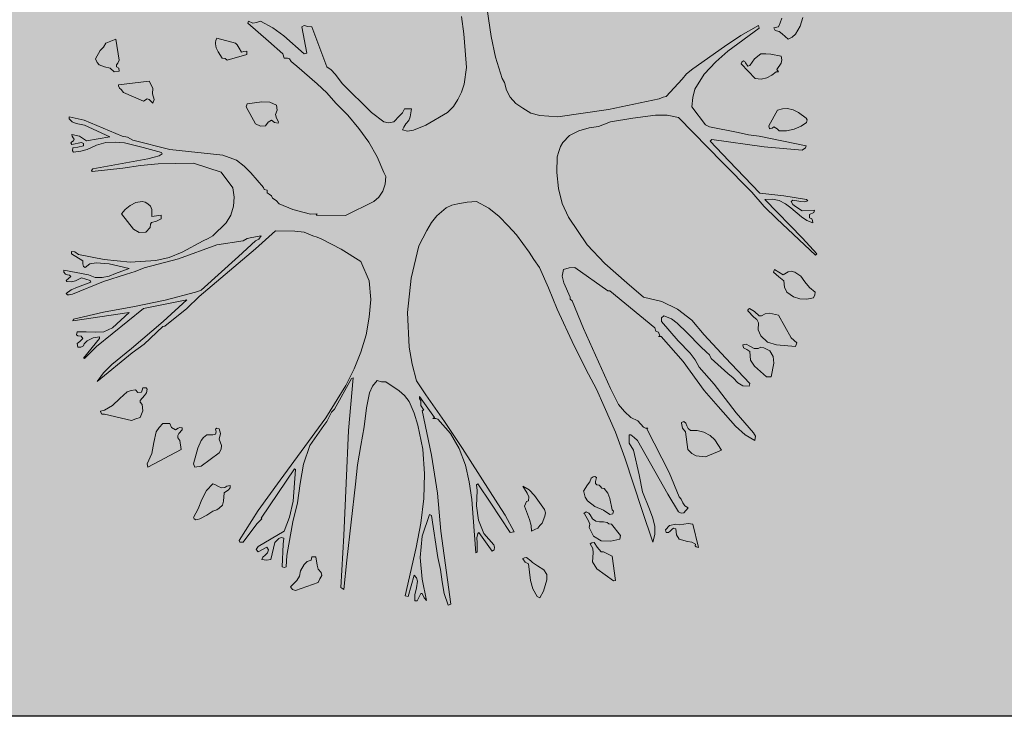
# Model space of a CAD drawing. Units: inches. Extents: x 84 to 1044, y -280 to 906.
# Tile 35 of 105: x 848 to 876, y -113 to -93. Entities that reach past the tile are written whole.
import ezdxf

# ---------------------------------------------------------------- set-up
doc = ezdxf.new("R2010")
doc.units = ezdxf.units.IN
doc.layers.add('C-PROP', color=7, linetype='Continuous', lineweight=25)
doc.layers.add('L-PLNT', color=114, linetype='Continuous', lineweight=15)
doc.layers.add('L-PLNT-PATT', color=9, linetype='Continuous', lineweight=9, true_color=0xafd9aa)

# ---------------------------------------------------------------- blocks, each defined once
blk = doc.blocks.new('A$C37E508DF')
for p, q in [((0.7911, 1.1436), (0.8027, 1.0677)), ((0.3456, 1.093), (0.3469, 1.0964)), ((0.3842, 1.0591), (0.3456, 1.093)), ((0.3469, 1.0964), (0.355, 1.093)), ((0.355, 1.093), (0.3619, 1.0943)), ((0.3619, 1.0943), (0.3692, 1.0968)), ((0.3692, 1.0968), (0.3923, 1.0844)), ((0.7512, 1.0728), (0.7469, 1.1054)), ((1.3421, 1.0861), (1.3455, 1.0934)), ((1.3455, 1.0934), (1.3485, 1.102)), ((1.3875, 1.1037), (1.3828, 1.087)), ((0.3923, 1.0844), (0.4129, 1.069)), ((0.4472, 1.0857), (0.4515, 1.0887)), ((0.4562, 1.0364), (0.4472, 1.0857)), ((0.4515, 1.0887), (0.4584, 1.0865)), ((0.4584, 1.0865), (0.4657, 1.0861)), ((0.4657, 1.0861), (0.4939, 1.0107)), ((0.7538, 1.0415), (0.7512, 1.0728)), ((1.3057, 1.0835), (1.2469, 1.0402)), ((1.2713, 1.0694), (1.3044, 1.0887)), ((1.3044, 1.0887), (1.3057, 1.0835)), ((1.3335, 1.0844), (1.3421, 1.0861)), ((1.3361, 1.0793), (1.3335, 1.0844)), ((1.3434, 1.0771), (1.3361, 1.0793)), ((1.349, 1.0728), (1.3434, 1.0771)), ((1.3605, 1.063), (1.349, 1.0728)), ((1.3828, 1.087), (1.3738, 1.072)), ((0.0746, 1.0475), (0.0789, 1.0552)), ((0.0789, 1.0552), (0.0978, 1.063)), ((0.0978, 1.063), (0.1042, 1.0231)), ((0.2847, 1.0565), (0.2856, 1.0604)), ((0.2851, 1.054), (0.2847, 1.0565)), ((0.2864, 1.0463), (0.2851, 1.054)), ((0.2856, 1.0604), (0.2877, 1.0647)), ((0.2877, 1.0647), (0.3224, 1.0552)), ((0.3224, 1.0552), (0.3255, 1.0522)), ((0.4112, 1.0351), (0.3842, 1.0591)), ((0.4129, 1.069), (0.4515, 1.0351)), ((0.8027, 1.0677), (0.8108, 1.0287)), ((1.2409, 1.0488), (1.2713, 1.0694)), ((1.3678, 1.0664), (1.3605, 1.063)), ((1.3738, 1.072), (1.3678, 1.0664)), ((0.0596, 1.0257), (0.0682, 1.0415)), ((0.0682, 1.0415), (0.0746, 1.0475)), ((0.2899, 1.039), (0.2864, 1.0463)), ((0.2972, 1.0274), (0.2899, 1.039)), ((0.3255, 1.0522), (0.3293, 1.0458)), ((0.3293, 1.0458), (0.3336, 1.0381)), ((0.3336, 1.0381), (0.3383, 1.0398)), ((0.3383, 1.0398), (0.3439, 1.0402)), ((0.3439, 1.0402), (0.3439, 1.0338)), ((0.4515, 1.0351), (0.4562, 1.0364)), ((0.7559, 1.0098), (0.7538, 1.0415)), ((1.1813, 1.0072), (1.2409, 1.0488)), ((1.2469, 1.0402), (1.2246, 1.0201)), ((1.3091, 1.0351), (1.3185, 1.0355)), ((1.3185, 1.0355), (1.3275, 1.0347)), ((0.0626, 1.0188), (0.0596, 1.0257)), ((0.0665, 1.0149), (0.0626, 1.0188)), ((0.1012, 1.018), (0.099, 1.0149)), ((0.1042, 1.0231), (0.1012, 1.018)), ((0.3032, 1.0265), (0.2972, 1.0274)), ((0.3066, 1.0231), (0.3032, 1.0265)), ((0.3439, 1.0338), (0.3066, 1.0231)), ((0.4138, 1.0274), (0.4112, 1.0351)), ((0.4202, 1.0274), (0.4138, 1.0274)), ((0.4241, 1.0257), (0.4202, 1.0274)), ((0.4267, 1.0209), (0.4241, 1.0257)), ((0.4305, 1.0175), (0.4267, 1.0209)), ((0.4378, 1.0124), (0.4305, 1.0175)), ((0.8108, 1.0287), (0.8233, 0.9892)), ((1.2246, 1.0201), (1.2023, 0.9969)), ((1.2718, 1.0162), (1.2731, 1.0197)), ((1.2731, 1.0197), (1.2761, 1.0218)), ((1.2761, 1.0218), (1.2786, 1.0209)), ((1.2786, 1.0209), (1.2799, 1.0184)), ((1.2799, 1.0184), (1.2842, 1.0124)), ((1.2885, 1.0136), (1.2971, 1.0257)), ((1.2971, 1.0257), (1.3091, 1.0351)), ((1.3275, 1.0347), (1.3468, 1.0308)), ((1.3468, 1.018), (1.3391, 1.0059)), ((1.3468, 1.0308), (1.3481, 1.0239)), ((1.3481, 1.0239), (1.3468, 1.018)), ((0.0763, 1.0111), (0.0665, 1.0149)), ((0.087, 1.0085), (0.0763, 1.0111)), ((0.0948, 1.0016), (0.087, 1.0085)), ((0.1042, 1.0029), (0.0948, 1.0016)), ((0.099, 1.0149), (0.099, 1.0111)), ((0.099, 1.0111), (0.1033, 1.0085)), ((0.1033, 1.0085), (0.1042, 1.0029)), ((0.476, 0.9789), (0.4378, 1.0124)), ((0.4939, 1.0107), (0.5021, 1.0051)), ((0.5021, 1.0051), (0.5094, 0.9969)), ((0.7516, 0.9785), (0.7559, 1.0098)), ((1.1693, 0.9974), (1.1813, 1.0072)), ((1.2984, 0.9892), (1.2718, 1.0162)), ((1.2842, 1.0124), (1.2885, 1.0136)), ((1.3378, 1.0016), (1.3297, 0.9952)), ((1.3421, 1.0016), (1.3378, 1.0016)), ((1.3391, 1.0059), (1.3421, 1.0016)), ((0.1029, 0.9772), (0.1604, 0.9841)), ((0.1604, 0.9841), (0.1672, 0.9708)), ((0.5094, 0.9969), (0.5231, 0.9789)), ((0.8233, 0.9892), (0.8275, 0.9815)), ((0.8275, 0.9815), (0.8314, 0.9673)), ((1.1311, 0.9549), (1.1612, 0.9879)), ((1.1612, 0.9879), (1.1693, 0.9974)), ((1.2023, 0.9969), (1.1852, 0.9691)), ((1.3095, 0.9875), (1.2984, 0.9892)), ((1.3202, 0.9901), (1.3095, 0.9875)), ((1.3297, 0.9952), (1.3202, 0.9901)), ((0.1025, 0.9751), (0.1029, 0.9772)), ((0.1046, 0.9708), (0.1025, 0.9751)), ((0.1076, 0.9682), (0.1046, 0.9708)), ((0.1119, 0.9626), (0.1076, 0.9682)), ((0.1496, 0.9463), (0.1119, 0.9626)), ((0.1672, 0.9708), (0.1664, 0.9601)), ((0.4939, 0.9618), (0.476, 0.9789)), ((0.5111, 0.9429), (0.4939, 0.9618)), ((0.5231, 0.9789), (0.578, 0.9253)), ((0.7401, 0.9493), (0.7469, 0.9635)), ((0.7469, 0.9635), (0.7516, 0.9785)), ((0.8314, 0.9673), (0.8383, 0.954)), ((1.1852, 0.9691), (1.1809, 0.9532)), ((0.1565, 0.9506), (0.1496, 0.9463)), ((0.1604, 0.9493), (0.1565, 0.9506)), ((0.1629, 0.9468), (0.1604, 0.9493)), ((0.1672, 0.9429), (0.1629, 0.9468)), ((0.1664, 0.9601), (0.1698, 0.9493)), ((0.1698, 0.9493), (0.1672, 0.9429)), ((0.3443, 0.9412), (0.3722, 0.9451)), ((0.3722, 0.9451), (0.3868, 0.9446)), ((0.3868, 0.9446), (0.3992, 0.9386)), ((0.7315, 0.9365), (0.7401, 0.9493)), ((0.8383, 0.954), (0.8486, 0.942)), ((1.0227, 0.9309), (1.1183, 0.9506)), ((1.1183, 0.9506), (1.1256, 0.954)), ((1.1256, 0.954), (1.1311, 0.9549)), ((1.1809, 0.9532), (1.1796, 0.936)), ((0.3426, 0.936), (0.3443, 0.9412)), ((0.3602, 0.9039), (0.3426, 0.936)), ((0.4009, 0.9292), (0.3975, 0.9215)), ((0.3992, 0.9386), (0.4009, 0.9292)), ((0.5334, 0.9202), (0.5111, 0.9429)), ((0.578, 0.9253), (0.6011, 0.9077)), ((0.6303, 0.9189), (0.6359, 0.9245)), ((0.6359, 0.9245), (0.6397, 0.9322)), ((0.6397, 0.9322), (0.653, 0.9322)), ((0.653, 0.9322), (0.6505, 0.9172)), ((0.6796, 0.9013), (0.7203, 0.9253)), ((0.7203, 0.9253), (0.7315, 0.9365)), ((0.8486, 0.942), (0.8619, 0.933)), ((0.8619, 0.933), (0.8769, 0.9236)), ((0.9279, 0.9172), (1.0227, 0.9309)), ((1.1796, 0.936), (1.2049, 0.9022)), ((1.3241, 0.9), (1.3404, 0.9292)), ((1.3404, 0.9292), (1.3494, 0.9322)), ((1.3494, 0.9322), (1.3592, 0.9326)), ((1.3592, 0.9326), (1.3695, 0.93)), ((1.3695, 0.93), (1.3794, 0.9253)), ((1.3794, 0.9253), (1.394, 0.9146)), ((0.0103, 0.9129), (0.0103, 0.9172)), ((0.0103, 0.9172), (0.0382, 0.9107)), ((0.0159, 0.9073), (0.0103, 0.9129)), ((0.0232, 0.9043), (0.0159, 0.9073)), ((0.0382, 0.9107), (0.1098, 0.8807)), ((0.3838, 0.9069), (0.379, 0.9)), ((0.3898, 0.9107), (0.3838, 0.9069)), ((0.3958, 0.906), (0.3898, 0.9107)), ((0.4026, 0.9052), (0.3958, 0.906)), ((0.3975, 0.9215), (0.3996, 0.9142)), ((0.3996, 0.9142), (0.4031, 0.9077)), ((0.4031, 0.9077), (0.4026, 0.9052)), ((0.554, 0.8953), (0.5334, 0.9202)), ((0.6011, 0.9077), (0.6097, 0.9056)), ((0.6097, 0.9056), (0.6196, 0.9077)), ((0.6196, 0.9077), (0.6303, 0.9189)), ((0.6479, 0.9103), (0.6423, 0.9039)), ((0.6505, 0.9172), (0.6479, 0.9103)), ((0.8769, 0.9236), (0.8936, 0.9193)), ((0.8936, 0.9193), (0.9279, 0.9172)), ((1.0269, 0.9077), (1.0042, 0.8987)), ((1.0685, 0.9142), (1.0269, 0.9077)), ((1.1114, 0.9198), (1.0685, 0.9142)), ((1.1333, 0.9202), (1.1114, 0.9198)), ((1.1543, 0.9159), (1.1333, 0.9202)), ((1.2371, 0.8314), (1.1543, 0.9159)), ((1.3948, 0.9065), (1.3846, 0.8992)), ((1.394, 0.9146), (1.3957, 0.9112)), ((1.3957, 0.9112), (1.3948, 0.9065)), ((0.0386, 0.9013), (0.0232, 0.9043)), ((0.0866, 0.8794), (0.0386, 0.9013)), ((0.3692, 0.8992), (0.3602, 0.9039)), ((0.379, 0.9), (0.3692, 0.8992)), ((0.5728, 0.8691), (0.554, 0.8953)), ((0.6384, 0.8974), (0.6359, 0.8927)), ((0.6359, 0.8927), (0.6457, 0.8897)), ((0.6423, 0.9039), (0.6384, 0.8974)), ((0.6457, 0.8897), (0.6569, 0.8919)), ((0.6569, 0.8919), (0.6796, 0.9013)), ((0.9673, 0.8906), (0.9498, 0.8816)), ((0.9866, 0.8962), (0.9673, 0.8906)), ((1.0042, 0.8987), (0.9866, 0.8962)), ((1.2049, 0.9022), (1.2126, 0.8983)), ((1.2126, 0.8983), (1.2662, 0.8876)), ((1.2662, 0.8876), (1.2855, 0.8833)), ((1.3254, 0.8944), (1.3241, 0.9)), ((1.3301, 0.8957), (1.3254, 0.8944)), ((1.3335, 0.8983), (1.3301, 0.8957)), ((1.3395, 0.8944), (1.3335, 0.8983)), ((1.3434, 0.8906), (1.3395, 0.8944)), ((1.3571, 0.8906), (1.3434, 0.8906)), ((1.3713, 0.8936), (1.3571, 0.8906)), ((1.3846, 0.8992), (1.3713, 0.8936)), ((0.0133, 0.8679), (0.015, 0.87)), ((0.015, 0.87), (0.0184, 0.8717)), ((0.0159, 0.8803), (0.0154, 0.8837)), ((0.0154, 0.8837), (0.0292, 0.8803)), ((0.0176, 0.8777), (0.0159, 0.8803)), ((0.0193, 0.8752), (0.0176, 0.8777)), ((0.0184, 0.8717), (0.0193, 0.8752)), ((0.0292, 0.8803), (0.0424, 0.8717)), ((0.0424, 0.8717), (0.0866, 0.8794)), ((0.0965, 0.8696), (0.0789, 0.8687)), ((0.1141, 0.8679), (0.0965, 0.8696)), ((0.1098, 0.8807), (0.1196, 0.8786)), ((0.1196, 0.8786), (0.1295, 0.873)), ((0.1295, 0.873), (0.1994, 0.8554)), ((0.5887, 0.8421), (0.5728, 0.8691)), ((0.9498, 0.8816), (0.9369, 0.8687)), ((1.2169, 0.8743), (1.2135, 0.8713)), ((1.2135, 0.8713), (1.2491, 0.834)), ((1.3151, 0.8606), (1.2169, 0.8743)), ((1.2855, 0.8833), (1.3057, 0.8807)), ((1.3057, 0.8807), (1.394, 0.8623)), ((0.0154, 0.8649), (0.0133, 0.8679)), ((0.0334, 0.8687), (0.0154, 0.8649)), ((0.0163, 0.8529), (0.0171, 0.8584)), ((0.0184, 0.8503), (0.0163, 0.8529)), ((0.0171, 0.8584), (0.0266, 0.8602)), ((0.0317, 0.8524), (0.0184, 0.8503)), ((0.0266, 0.8602), (0.0369, 0.8623)), ((0.0442, 0.8554), (0.0317, 0.8524)), ((0.0369, 0.8666), (0.0334, 0.8687)), ((0.0369, 0.8623), (0.0369, 0.8666)), ((0.0617, 0.864), (0.0442, 0.8554)), ((0.0789, 0.8687), (0.0617, 0.864)), ((0.1492, 0.8593), (0.1141, 0.8679)), ((0.1835, 0.8499), (0.1492, 0.8593)), ((0.1994, 0.8554), (0.2984, 0.8447)), ((0.9296, 0.852), (0.9262, 0.8421)), ((0.933, 0.861), (0.9296, 0.852)), ((0.9369, 0.8687), (0.933, 0.861)), ((1.3863, 0.8541), (1.3151, 0.8606)), ((1.3927, 0.8584), (1.3863, 0.8541)), ((1.394, 0.8623), (1.3927, 0.8584)), ((0.0545, 0.8194), (0.1578, 0.8378)), ((0.1578, 0.8378), (0.1698, 0.8413)), ((0.1698, 0.8413), (0.1792, 0.8434)), ((0.1792, 0.8434), (0.1848, 0.8477)), ((0.1848, 0.8477), (0.1835, 0.8499)), ((0.2984, 0.8447), (0.3242, 0.8357)), ((0.3242, 0.8357), (0.3387, 0.8241)), ((0.6007, 0.8125), (0.5887, 0.8421)), ((0.9262, 0.8421), (0.9257, 0.8121)), ((1.2491, 0.834), (1.3069, 0.7735)), ((0.0519, 0.8164), (0.0545, 0.8194)), ((0.0532, 0.8143), (0.0519, 0.8164)), ((0.1111, 0.8207), (0.0532, 0.8143)), ((0.1441, 0.8258), (0.1111, 0.8207)), ((0.1771, 0.8288), (0.1441, 0.8258)), ((0.2436, 0.8301), (0.1771, 0.8288)), ((0.2954, 0.813), (0.2436, 0.8301)), ((0.3387, 0.8241), (0.3512, 0.8117)), ((1.2919, 0.7752), (1.2371, 0.8314)), ((0.3173, 0.7834), (0.2954, 0.813)), ((0.3512, 0.8117), (0.3748, 0.7842)), ((0.6046, 0.8048), (0.6007, 0.8125)), ((0.6037, 0.7903), (0.6046, 0.8048)), ((0.9257, 0.8121), (0.9287, 0.7825)), ((0.3199, 0.7662), (0.3173, 0.7834)), ((0.3748, 0.7842), (0.3765, 0.7804)), ((0.3765, 0.7804), (0.3816, 0.7791)), ((0.3816, 0.7791), (0.382, 0.7744)), ((0.5913, 0.7658), (0.599, 0.777)), ((0.599, 0.777), (0.6037, 0.7903)), ((0.9287, 0.7825), (0.936, 0.7542)), ((0.3186, 0.7491), (0.3199, 0.7662)), ((0.382, 0.7744), (0.3859, 0.7714)), ((0.3859, 0.7714), (0.3902, 0.7684)), ((0.3902, 0.7684), (0.3919, 0.7641)), ((0.3919, 0.7641), (0.3988, 0.7598)), ((0.3988, 0.7598), (0.4043, 0.7538)), ((0.5823, 0.7577), (0.5913, 0.7658)), ((1.3151, 0.7487), (1.2919, 0.7752)), ((1.3069, 0.7735), (1.352, 0.7684)), ((1.3309, 0.7624), (1.3164, 0.7615)), ((1.3164, 0.7615), (1.3871, 0.6891)), ((1.3434, 0.7598), (1.3309, 0.7624)), ((1.355, 0.7538), (1.3434, 0.7598)), ((1.352, 0.7684), (1.3948, 0.7615)), ((1.3687, 0.7607), (1.3657, 0.7577)), ((1.3841, 0.7577), (1.3687, 0.7607)), ((1.397, 0.759), (1.3914, 0.7572)), ((1.3948, 0.7615), (1.397, 0.759)), ((0.1081, 0.7349), (0.1153, 0.7427)), ((0.1153, 0.7427), (0.1244, 0.7504)), ((0.1244, 0.7504), (0.1351, 0.7559)), ((0.1351, 0.7559), (0.1471, 0.7577)), ((0.1471, 0.7577), (0.1527, 0.7568)), ((0.1527, 0.7568), (0.1578, 0.7538)), ((0.1578, 0.7538), (0.1629, 0.7491)), ((0.1629, 0.7491), (0.1651, 0.7431)), ((0.1651, 0.7431), (0.1655, 0.7298)), ((0.3139, 0.7324), (0.3186, 0.7491)), ((0.4043, 0.7538), (0.4301, 0.7431)), ((0.4301, 0.7431), (0.4515, 0.7371)), ((0.5287, 0.7319), (0.5823, 0.7577)), ((0.7182, 0.7461), (0.7002, 0.7307)), ((0.7285, 0.7512), (0.7182, 0.7461)), ((0.7401, 0.7534), (0.7285, 0.7512)), ((0.7577, 0.7568), (0.7401, 0.7534)), ((0.7752, 0.7577), (0.7577, 0.7568)), ((0.798, 0.7452), (0.7752, 0.7577)), ((0.8173, 0.7298), (0.798, 0.7452)), ((0.936, 0.7542), (0.9476, 0.7285)), ((1.3391, 0.7255), (1.3151, 0.7487)), ((1.3653, 0.7461), (1.355, 0.7538)), ((1.3854, 0.7294), (1.3653, 0.7461)), ((1.3657, 0.7577), (1.3691, 0.7521)), ((1.3691, 0.7521), (1.3743, 0.7482)), ((1.3743, 0.7482), (1.3863, 0.7405)), ((1.3914, 0.7572), (1.3841, 0.7577)), ((1.3863, 0.7405), (1.4099, 0.7414)), ((1.4099, 0.7414), (1.4086, 0.7375)), ((0.1312, 0.7058), (0.1081, 0.7349)), ((0.1655, 0.7298), (0.1831, 0.7324)), ((0.1831, 0.7255), (0.1741, 0.7208)), ((0.1831, 0.7324), (0.1831, 0.7255)), ((0.3049, 0.7178), (0.3139, 0.7324)), ((0.4515, 0.7371), (0.4635, 0.7341)), ((0.4635, 0.7341), (0.4755, 0.7349)), ((0.4755, 0.7349), (0.4742, 0.7324)), ((0.4742, 0.7324), (0.5287, 0.7319)), ((0.7002, 0.7307), (0.6903, 0.7186)), ((0.8344, 0.7122), (0.8173, 0.7298)), ((0.9476, 0.7285), (0.9828, 0.6762)), ((1.4116, 0.6569), (1.3391, 0.7255)), ((1.3953, 0.7221), (1.3854, 0.7294)), ((1.4064, 0.7178), (1.3953, 0.7221)), ((1.4086, 0.7375), (1.4004, 0.7337)), ((1.4004, 0.7337), (1.4004, 0.7272)), ((1.4004, 0.7272), (1.4047, 0.7255)), ((1.4047, 0.7255), (1.406, 0.7221)), ((1.406, 0.7221), (1.4064, 0.7178)), ((0.1415, 0.6994), (0.1312, 0.7058)), ((0.1621, 0.7092), (0.1539, 0.7002)), ((0.1629, 0.7152), (0.1621, 0.7092)), ((0.1646, 0.7186), (0.1629, 0.7152)), ((0.1741, 0.7208), (0.1646, 0.7186)), ((0.28, 0.6933), (0.3049, 0.7178)), ((0.3975, 0.7028), (0.3598, 0.6693)), ((0.4339, 0.7019), (0.3975, 0.7028)), ((0.6818, 0.7032), (0.6667, 0.6749)), ((0.6903, 0.7186), (0.6818, 0.7032)), ((0.8503, 0.6951), (0.8344, 0.7122)), ((0.1539, 0.7002), (0.1415, 0.6994)), ((0.262, 0.6839), (0.271, 0.6882)), ((0.271, 0.6882), (0.28, 0.6933)), ((0.337, 0.6843), (0.2877, 0.6762)), ((0.328, 0.6543), (0.3598, 0.6843)), ((0.3443, 0.6886), (0.337, 0.6843)), ((0.3533, 0.6903), (0.3443, 0.6886)), ((0.3709, 0.6933), (0.3533, 0.6903)), ((0.3598, 0.6843), (0.3662, 0.6873)), ((0.3662, 0.6873), (0.3709, 0.6933)), ((0.4515, 0.7002), (0.4339, 0.7019)), ((0.4674, 0.6933), (0.4515, 0.7002)), ((0.476, 0.6912), (0.4674, 0.6933)), ((0.4832, 0.6878), (0.476, 0.6912)), ((0.521, 0.6685), (0.4832, 0.6878)), ((0.8739, 0.6629), (0.8503, 0.6951)), ((1.3871, 0.6891), (1.4141, 0.6599)), ((0.2877, 0.6762), (0.2152, 0.6505)), ((0.2221, 0.6625), (0.262, 0.6839)), ((0.3598, 0.6693), (0.2543, 0.5797)), ((0.5578, 0.6449), (0.521, 0.6685)), ((0.6667, 0.6749), (0.6526, 0.614)), ((0.9828, 0.6762), (1.0162, 0.6415)), ((0.0146, 0.6599), (0.0146, 0.6642)), ((0.0146, 0.6642), (0.0206, 0.6633)), ((0.036, 0.6466), (0.0146, 0.6599)), ((0.0206, 0.6633), (0.0274, 0.6586)), ((0.0274, 0.6586), (0.0759, 0.6492)), ((0.0759, 0.6492), (0.1244, 0.644)), ((0.2152, 0.6505), (0.1509, 0.6333)), ((0.1728, 0.647), (0.1977, 0.6526)), ((0.1977, 0.6526), (0.2221, 0.6625)), ((0.2581, 0.5913), (0.328, 0.6543)), ((0.8824, 0.6492), (0.8739, 0.6629)), ((0.8932, 0.6342), (0.8824, 0.6492)), ((1.4141, 0.6599), (1.4116, 0.6569)), ((0, 0.629), (0.0467, 0.62)), ((0, 0.6252), (0, 0.629)), ((0.0356, 0.6406), (0.036, 0.6466)), ((0.0369, 0.6355), (0.0356, 0.6406)), ((0.0399, 0.6342), (0.0369, 0.6355)), ((0.0489, 0.641), (0.0399, 0.6342)), ((0.0609, 0.6428), (0.0489, 0.641)), ((0.0853, 0.641), (0.0609, 0.6428)), ((0.1226, 0.632), (0.0853, 0.641)), ((0.0973, 0.6226), (0.1226, 0.632)), ((0.1244, 0.644), (0.1728, 0.647)), ((0.1509, 0.6333), (0.1342, 0.6265)), ((0.5737, 0.6089), (0.5578, 0.6449)), ((0.9103, 0.5956), (0.8932, 0.6342)), ((0.9382, 0.6303), (0.936, 0.6179)), ((0.9493, 0.6333), (0.9382, 0.6303)), ((0.9596, 0.6342), (0.9493, 0.6333)), ((1.0218, 0.5904), (0.9596, 0.6342)), ((1.0162, 0.6415), (1.0574, 0.605)), ((1.3327, 0.6252), (1.3348, 0.6303)), ((1.3348, 0.6303), (1.3511, 0.62)), ((0.003, 0.6213), (0, 0.6252)), ((0.0069, 0.6204), (0.003, 0.6213)), ((0.0047, 0.6093), (0.0086, 0.6132)), ((0.0107, 0.6196), (0.0069, 0.6204)), ((0.0086, 0.6132), (0.0133, 0.617)), ((0.0133, 0.617), (0.0107, 0.6196)), ((0.0334, 0.6145), (0.0223, 0.6089)), ((0.0416, 0.6119), (0.0334, 0.6145)), ((0.0493, 0.6093), (0.0416, 0.6119)), ((0.0467, 0.62), (0.0592, 0.6153)), ((0.0592, 0.6153), (0.072, 0.6149)), ((0.072, 0.6149), (0.0849, 0.6175)), ((0.1175, 0.6213), (0.0746, 0.6076)), ((0.0849, 0.6175), (0.0973, 0.6226)), ((0.1342, 0.6265), (0.1175, 0.6213)), ((0.6526, 0.614), (0.6457, 0.5497)), ((0.936, 0.6179), (0.939, 0.605)), ((1.343, 0.6162), (1.3327, 0.6252)), ((1.352, 0.6089), (1.343, 0.6162)), ((1.3511, 0.62), (1.3601, 0.6256)), ((1.3601, 0.6256), (1.3661, 0.6269)), ((1.3661, 0.6269), (1.3725, 0.6252)), ((1.3725, 0.6252), (1.3837, 0.6175)), ((1.3837, 0.6175), (1.3918, 0.6072)), ((0.0056, 0.6076), (0.0047, 0.6093)), ((0.0047, 0.5849), (0.0141, 0.5921)), ((0.0141, 0.6072), (0.0056, 0.6076)), ((0.0223, 0.6089), (0.0141, 0.6072)), ((0.0141, 0.5921), (0.0257, 0.5969)), ((0.0746, 0.6076), (0.0163, 0.5836)), ((0.0257, 0.5969), (0.0506, 0.6063)), ((0.0506, 0.6063), (0.0493, 0.6093)), ((0.5763, 0.5741), (0.5737, 0.6089)), ((0.9262, 0.5557), (0.9103, 0.5956)), ((0.939, 0.605), (0.9506, 0.5784)), ((1.0574, 0.605), (1.0883, 0.5784)), ((1.3533, 0.5969), (1.352, 0.6089)), ((1.358, 0.5874), (1.3533, 0.5969)), ((1.3918, 0.6072), (1.4004, 0.5964)), ((1.4004, 0.5964), (1.4111, 0.5874)), ((0.0069, 0.5823), (0.0047, 0.5849)), ((0.0099, 0.5823), (0.0069, 0.5823)), ((0.0163, 0.5836), (0.0099, 0.5823)), ((0.1904, 0.5724), (0.2474, 0.5879)), ((0.2543, 0.5797), (0.2311, 0.557)), ((0.2474, 0.5879), (0.253, 0.5892)), ((0.253, 0.5892), (0.2581, 0.5913)), ((0.5737, 0.5407), (0.5763, 0.5741)), ((0.9506, 0.5784), (0.951, 0.5746)), ((0.951, 0.5746), (0.9545, 0.5711)), ((1.0256, 0.5904), (1.0218, 0.5904)), ((1.1097, 0.5205), (1.0256, 0.5904)), ((1.0883, 0.5784), (1.123, 0.5703)), ((1.37, 0.5789), (1.358, 0.5874)), ((1.3824, 0.575), (1.37, 0.5789)), ((1.3953, 0.5746), (1.3824, 0.575)), ((1.4077, 0.5771), (1.3953, 0.5746)), ((1.4103, 0.5823), (1.4077, 0.5771)), ((1.4111, 0.5874), (1.4103, 0.5823)), ((0.1496, 0.557), (0.0613, 0.4858)), ((0.0746, 0.5501), (0.1325, 0.5608)), ((0.1325, 0.5608), (0.1904, 0.5724)), ((0.2311, 0.5729), (0.1496, 0.557)), ((0.1869, 0.5325), (0.2311, 0.5729)), ((0.2311, 0.557), (0.1899, 0.5235)), ((0.9583, 0.4871), (0.9262, 0.5557)), ((0.9545, 0.5711), (0.9759, 0.5193)), ((1.123, 0.5703), (1.1526, 0.5557)), ((1.1526, 0.5557), (1.1792, 0.5347)), ((1.2842, 0.554), (1.2855, 0.5557)), ((1.2855, 0.5557), (1.2876, 0.557)), ((1.2876, 0.557), (1.2971, 0.551)), ((0.1226, 0.5497), (0.0171, 0.5338)), ((0.0171, 0.5338), (0.0184, 0.5368)), ((0.0184, 0.5368), (0.0746, 0.5501)), ((0.0917, 0.5205), (0.1226, 0.5497)), ((0.5677, 0.5077), (0.5737, 0.5407)), ((0.6457, 0.5497), (0.6483, 0.4845)), ((1.1226, 0.5394), (1.1221, 0.5325)), ((1.1268, 0.5433), (1.1226, 0.5394)), ((1.141, 0.5377), (1.1268, 0.5433)), ((1.1521, 0.5296), (1.141, 0.5377)), ((1.2842, 0.5527), (1.2842, 0.554)), ((1.2958, 0.5407), (1.2842, 0.5527)), ((1.3014, 0.536), (1.2958, 0.5407)), ((1.2971, 0.551), (1.3057, 0.5433)), ((1.3057, 0.5433), (1.3099, 0.5433)), ((1.3099, 0.5433), (1.3172, 0.5467)), ((1.3172, 0.5467), (1.3254, 0.548)), ((1.3254, 0.548), (1.3421, 0.5446)), ((1.3421, 0.5446), (1.3657, 0.5021)), ((0.0755, 0.5133), (0.0917, 0.5205)), ((0.1269, 0.482), (0.1869, 0.5325)), ((0.1861, 0.5231), (0.1509, 0.4897)), ((0.1899, 0.5235), (0.1861, 0.5231)), ((0.9759, 0.5193), (1.0269, 0.4069)), ((1.1118, 0.5145), (1.1097, 0.5205)), ((1.1221, 0.5325), (1.1539, 0.4961)), ((1.1706, 0.5111), (1.1521, 0.5296)), ((1.1792, 0.5347), (1.2027, 0.5072)), ((1.3044, 0.53), (1.3014, 0.536)), ((1.3039, 0.5167), (1.3044, 0.53)), ((0.024, 0.5072), (0.0253, 0.5128)), ((0.0262, 0.5055), (0.024, 0.5072)), ((0.0253, 0.5128), (0.042, 0.5133)), ((0.0326, 0.5047), (0.0262, 0.5055)), ((0.03, 0.4948), (0.036, 0.5004)), ((0.036, 0.5004), (0.0326, 0.5047)), ((0.0369, 0.4639), (0.0669, 0.5004)), ((0.042, 0.5133), (0.0587, 0.5124)), ((0.0549, 0.5021), (0.0437, 0.4961)), ((0.0669, 0.5034), (0.0549, 0.5021)), ((0.0587, 0.5124), (0.0755, 0.5133)), ((0.0669, 0.5004), (0.0669, 0.5034)), ((0.5578, 0.4751), (0.5677, 0.5077)), ((1.117, 0.5124), (1.1118, 0.5145)), ((1.1191, 0.5055), (1.117, 0.5124)), ((1.117, 0.5042), (1.1191, 0.5055)), ((1.1217, 0.5042), (1.117, 0.5042)), ((1.1633, 0.4575), (1.1217, 0.5042)), ((1.1955, 0.4858), (1.1706, 0.5111)), ((1.2027, 0.5072), (1.2426, 0.4644)), ((1.3091, 0.5055), (1.3039, 0.5167)), ((1.3215, 0.4935), (1.3091, 0.5055)), ((1.3657, 0.5021), (1.3764, 0.4927)), ((0.0253, 0.491), (0.03, 0.4948)), ((0.0262, 0.4841), (0.0253, 0.491)), ((0.0317, 0.4841), (0.0262, 0.4841)), ((0.0369, 0.4871), (0.0317, 0.4841)), ((0.0382, 0.4905), (0.0369, 0.4871)), ((0.0403, 0.4922), (0.0382, 0.4905)), ((0.0613, 0.4858), (0.0386, 0.4627)), ((0.0437, 0.4961), (0.0403, 0.4922)), ((0.0905, 0.4515), (0.1269, 0.482)), ((0.1509, 0.4897), (0.1282, 0.4734)), ((0.6483, 0.4845), (0.6539, 0.4524)), ((0.9853, 0.4335), (0.9583, 0.4871)), ((1.1539, 0.4961), (1.1762, 0.4729)), ((1.207, 0.4747), (1.1955, 0.4858)), ((1.2748, 0.4884), (1.2812, 0.4897)), ((1.2761, 0.4832), (1.2748, 0.4884)), ((1.2825, 0.4798), (1.2761, 0.4832)), ((1.2812, 0.4897), (1.2885, 0.4862)), ((1.2885, 0.4862), (1.2962, 0.4815)), ((1.2962, 0.4815), (1.3039, 0.482)), ((1.3039, 0.482), (1.3087, 0.4841)), ((1.3087, 0.4841), (1.3147, 0.4832)), ((1.3147, 0.4832), (1.3258, 0.4777)), ((1.3382, 0.4884), (1.3215, 0.4935)), ((1.3743, 0.4858), (1.3382, 0.4884)), ((1.3764, 0.4927), (1.3743, 0.4858)), ((0.0386, 0.4627), (0.0369, 0.4639)), ((0.1282, 0.4734), (0.0626, 0.4198)), ((0.545, 0.4434), (0.5578, 0.4751)), ((1.1762, 0.4729), (1.1856, 0.4605)), ((1.2122, 0.47), (1.207, 0.4747)), ((1.2156, 0.4627), (1.2122, 0.47)), ((1.2469, 0.4348), (1.2156, 0.4627)), ((1.2426, 0.4644), (1.2885, 0.4159)), ((1.2885, 0.4764), (1.2825, 0.4798)), ((1.2894, 0.4601), (1.2885, 0.4764)), ((1.3258, 0.4777), (1.3318, 0.4669)), ((1.3318, 0.4669), (1.3331, 0.4545)), ((0.0746, 0.4361), (0.0905, 0.4515)), ((0.6539, 0.4524), (0.6625, 0.4211)), ((1.2027, 0.4026), (1.1633, 0.4575)), ((1.1856, 0.4605), (1.1933, 0.4468)), ((1.1933, 0.4468), (1.2212, 0.4146)), ((1.2967, 0.4485), (1.2894, 0.4601)), ((1.3082, 0.4386), (1.2967, 0.4485)), ((1.3331, 0.4545), (1.3284, 0.4284)), ((0.0626, 0.4198), (0.0746, 0.4361)), ((0.5403, 0.4254), (0.5081, 0.3679)), ((0.5295, 0.4125), (0.545, 0.4434)), ((0.5347, 0.3276), (0.5433, 0.4266)), ((0.5433, 0.4266), (0.5403, 0.4254)), ((1.0003, 0.4052), (0.9853, 0.4335)), ((1.2568, 0.4266), (1.2469, 0.4348)), ((1.2658, 0.4176), (1.2568, 0.4266)), ((1.3198, 0.4284), (1.3082, 0.4386)), ((1.3284, 0.4284), (1.3198, 0.4284)), ((0.1471, 0.4035), (0.1484, 0.4082)), ((0.1484, 0.4082), (0.1548, 0.4082)), ((0.1548, 0.4082), (0.1565, 0.4052)), ((0.4922, 0.3516), (0.5295, 0.4125)), ((0.5797, 0.4112), (0.5741, 0.3983)), ((0.5887, 0.4215), (0.5797, 0.4112)), ((0.5969, 0.4189), (0.5887, 0.4215)), ((0.6046, 0.4189), (0.5969, 0.4189)), ((0.6295, 0.4022), (0.6046, 0.4189)), ((0.6625, 0.4211), (0.6796, 0.3945)), ((1.0269, 0.4069), (1.0419, 0.3769)), ((1.2212, 0.4146), (1.2628, 0.361)), ((1.2752, 0.4116), (1.2658, 0.4176)), ((1.2868, 0.4108), (1.2752, 0.4116)), ((1.2885, 0.4159), (1.2868, 0.4108)), ((0.1055, 0.388), (0.1192, 0.4001)), ((0.1192, 0.4001), (0.1265, 0.4031)), ((0.1265, 0.4031), (0.1346, 0.4039)), ((0.1346, 0.4039), (0.1389, 0.3992)), ((0.1389, 0.3992), (0.1458, 0.3996)), ((0.1518, 0.3932), (0.1432, 0.3842)), ((0.1458, 0.3996), (0.1471, 0.4035)), ((0.1556, 0.3983), (0.1518, 0.3932)), ((0.1565, 0.4052), (0.1556, 0.3983)), ((0.5741, 0.3983), (0.5686, 0.3705)), ((0.6397, 0.3936), (0.6295, 0.4022)), ((0.6487, 0.3825), (0.6397, 0.3936)), ((0.6959, 0.352), (0.668, 0.3919)), ((0.668, 0.3919), (0.668, 0.3872)), ((0.6796, 0.3945), (0.7148, 0.3447)), ((1.0145, 0.373), (1.0003, 0.4052)), ((1.2289, 0.373), (1.2027, 0.4026)), ((0.0763, 0.3662), (0.0917, 0.3748)), ((0.0917, 0.3748), (0.1055, 0.388)), ((0.1432, 0.3842), (0.1436, 0.3808)), ((0.1436, 0.3808), (0.1471, 0.3769)), ((0.1471, 0.3769), (0.1484, 0.3649)), ((0.5686, 0.3705), (0.5643, 0.3349)), ((0.6582, 0.3602), (0.6487, 0.3825)), ((0.668, 0.3872), (0.6706, 0.3842)), ((0.6706, 0.3842), (0.6702, 0.3748)), ((0.6702, 0.3748), (0.6762, 0.3662)), ((1.0359, 0.3246), (1.0145, 0.373)), ((1.0419, 0.3769), (1.0527, 0.3632)), ((1.2615, 0.3362), (1.2289, 0.373)), ((0.069, 0.364), (0.0763, 0.3662)), ((0.069, 0.3627), (0.069, 0.364)), ((0.0716, 0.3585), (0.069, 0.3627)), ((0.0763, 0.3585), (0.0716, 0.3585)), ((0.1269, 0.3464), (0.0763, 0.3585)), ((0.1432, 0.352), (0.1355, 0.3499)), ((0.1484, 0.3649), (0.1432, 0.352)), ((0.4065, 0.2345), (0.4922, 0.3516)), ((0.4982, 0.3537), (0.4939, 0.3447)), ((0.5025, 0.3619), (0.4982, 0.3537)), ((0.5081, 0.3679), (0.5025, 0.3619)), ((0.665, 0.3379), (0.6582, 0.3602)), ((0.6762, 0.3662), (0.6732, 0.3653)), ((0.6732, 0.3653), (0.6903, 0.2813)), ((0.6933, 0.3503), (0.6959, 0.352)), ((1.0527, 0.3632), (1.0647, 0.352)), ((1.0647, 0.352), (1.078, 0.346)), ((1.2628, 0.361), (1.2949, 0.3233)), ((0.1355, 0.3499), (0.1269, 0.3464)), ((0.1737, 0.325), (0.1788, 0.3336)), ((0.1788, 0.3336), (0.1861, 0.3409)), ((0.1861, 0.3409), (0.199, 0.3409)), ((0.199, 0.3409), (0.2024, 0.3336)), ((0.2024, 0.3336), (0.2097, 0.3289)), ((0.2148, 0.3323), (0.2182, 0.3336)), ((0.2182, 0.3336), (0.2221, 0.3327)), ((0.4884, 0.337), (0.4622, 0.2997)), ((0.4939, 0.3447), (0.4884, 0.337)), ((0.5643, 0.3349), (0.5578, 0.2993)), ((0.6745, 0.2924), (0.665, 0.3379)), ((0.6985, 0.3503), (0.6933, 0.3503)), ((0.7023, 0.349), (0.6985, 0.3503)), ((0.7259, 0.3224), (0.7023, 0.349)), ((0.7148, 0.3447), (0.7487, 0.2937)), ((1.078, 0.346), (1.0883, 0.334)), ((1.0883, 0.334), (1.0921, 0.3319)), ((1.1599, 0.3426), (1.1646, 0.3447)), ((1.1599, 0.3413), (1.1599, 0.3426)), ((1.162, 0.3319), (1.1599, 0.3413)), ((1.1646, 0.3447), (1.168, 0.3417)), ((1.168, 0.3417), (1.1702, 0.3366)), ((1.1702, 0.3366), (1.1727, 0.3314)), ((1.2795, 0.3199), (1.2615, 0.3362)), ((0.1689, 0.3053), (0.1737, 0.325)), ((0.2097, 0.3289), (0.2148, 0.3323)), ((0.2161, 0.3224), (0.214, 0.3186)), ((0.214, 0.3186), (0.214, 0.3139)), ((0.2221, 0.3289), (0.2161, 0.3224)), ((0.2221, 0.3327), (0.2221, 0.3289)), ((0.2577, 0.3087), (0.2624, 0.3147)), ((0.2624, 0.3147), (0.2689, 0.3194)), ((0.2689, 0.3194), (0.2796, 0.3194)), ((0.2796, 0.3194), (0.2847, 0.3211)), ((0.2847, 0.3211), (0.2864, 0.325)), ((0.2851, 0.3302), (0.2877, 0.3319)), ((0.2864, 0.325), (0.2851, 0.3302)), ((0.2877, 0.3319), (0.292, 0.3306)), ((0.292, 0.3306), (0.2941, 0.322)), ((0.2941, 0.322), (0.292, 0.3117)), ((0.53, 0.229), (0.5347, 0.3276)), ((0.7427, 0.2937), (0.7259, 0.3224)), ((1.0535, 0.2766), (1.0359, 0.3246)), ((1.0647, 0.3199), (1.0617, 0.3194)), ((1.0617, 0.3194), (1.0617, 0.304)), ((1.0711, 0.3147), (1.0647, 0.3199)), ((1.0775, 0.3092), (1.0711, 0.3147)), ((1.0921, 0.3319), (1.0968, 0.3319)), ((1.0968, 0.3319), (1.0947, 0.3306)), ((1.0947, 0.3306), (1.1367, 0.2491)), ((1.1676, 0.325), (1.162, 0.3319)), ((1.1719, 0.292), (1.1676, 0.325)), ((1.1727, 0.3314), (1.177, 0.3276)), ((1.177, 0.3276), (1.1895, 0.3276)), ((1.1895, 0.3276), (1.2019, 0.3246)), ((1.2019, 0.3246), (1.2135, 0.3186)), ((1.2135, 0.3186), (1.2225, 0.3104)), ((1.2975, 0.3087), (1.2795, 0.3199)), ((1.2949, 0.3233), (1.2988, 0.3173)), ((1.2988, 0.3173), (1.2975, 0.3087)), ((0.1655, 0.2843), (0.1689, 0.3053)), ((0.214, 0.3139), (0.2182, 0.3087)), ((0.2182, 0.3087), (0.2204, 0.292)), ((0.2517, 0.2946), (0.2577, 0.3087)), ((0.292, 0.3117), (0.2959, 0.2993)), ((0.2959, 0.2993), (0.2954, 0.2928)), ((0.4622, 0.2997), (0.4502, 0.2645)), ((0.5578, 0.2993), (0.5518, 0.2633)), ((1.0617, 0.304), (1.0698, 0.2911)), ((1.1341, 0.2084), (1.0775, 0.3092)), ((1.2225, 0.3104), (1.2349, 0.2911)), ((0.1565, 0.265), (0.1655, 0.2843)), ((0.2204, 0.292), (0.1578, 0.259)), ((0.2436, 0.265), (0.2517, 0.2946)), ((0.292, 0.286), (0.2581, 0.2607)), ((0.2954, 0.2928), (0.292, 0.286)), ((0.6775, 0.2465), (0.6745, 0.2924)), ((0.6903, 0.2813), (0.7015, 0.2101)), ((0.7542, 0.2628), (0.7427, 0.2937)), ((0.7487, 0.2937), (0.8151, 0.1899)), ((1.0698, 0.2911), (1.0805, 0.2448)), ((1.1792, 0.2847), (1.1719, 0.292)), ((1.1873, 0.28), (1.1792, 0.2847)), ((1.2049, 0.2783), (1.1873, 0.28)), ((1.2349, 0.2911), (1.2049, 0.2783)), ((0.1578, 0.259), (0.1565, 0.265)), ((0.2461, 0.259), (0.2436, 0.265)), ((0.2581, 0.2607), (0.2461, 0.259)), ((0.4502, 0.2645), (0.4438, 0.2285)), ((0.5518, 0.2633), (0.5475, 0.2268)), ((0.7615, 0.2311), (0.7542, 0.2628)), ((1.0861, 0.1775), (1.0535, 0.2766)), ((0.4335, 0.2556), (0.3709, 0.1634)), ((0.4305, 0.1951), (0.4352, 0.2543)), ((0.4352, 0.2543), (0.4335, 0.2556)), ((0.6758, 0.2002), (0.6775, 0.2465)), ((0.9905, 0.2384), (0.9943, 0.241)), ((0.9943, 0.241), (0.9973, 0.2414)), ((0.9973, 0.2414), (1.0003, 0.2393)), ((1.0805, 0.2448), (1.087, 0.2127)), ((1.1367, 0.2491), (1.1556, 0.2032)), ((0.268, 0.2148), (0.28, 0.2277)), ((0.28, 0.2277), (0.2851, 0.226)), ((0.2851, 0.226), (0.2903, 0.2225)), ((0.2903, 0.2225), (0.2963, 0.22)), ((0.3027, 0.2204), (0.3061, 0.2234)), ((0.3061, 0.2234), (0.3122, 0.2247)), ((0.3122, 0.2247), (0.3122, 0.22)), ((0.3649, 0.1775), (0.4065, 0.2345)), ((0.4438, 0.2285), (0.4391, 0.1921)), ((0.5261, 0.1308), (0.53, 0.229)), ((0.5475, 0.2268), (0.5313, 0.084)), ((0.7662, 0.1981), (0.7615, 0.2311)), ((0.7778, 0.2277), (0.7752, 0.2255)), ((0.7752, 0.2255), (0.7761, 0.2152)), ((0.8018, 0.1912), (0.7778, 0.2277)), ((0.8619, 0.2234), (0.8739, 0.2161)), ((0.87, 0.2101), (0.8619, 0.2234)), ((0.9759, 0.214), (0.9836, 0.226)), ((0.9836, 0.226), (0.9879, 0.2311)), ((0.9879, 0.2311), (0.9905, 0.2384)), ((1.0003, 0.2393), (0.9986, 0.232)), ((0.9986, 0.232), (0.9986, 0.2281)), ((0.9986, 0.2281), (1.0012, 0.2255)), ((1.0012, 0.2255), (1.0051, 0.2251)), ((1.0051, 0.2251), (1.0076, 0.2225)), ((1.0076, 0.2225), (1.0106, 0.2195)), ((0.2594, 0.1981), (0.268, 0.2148)), ((0.2963, 0.22), (0.3027, 0.2204)), ((0.301, 0.211), (0.3002, 0.1951)), ((0.3096, 0.2165), (0.301, 0.211)), ((0.3122, 0.22), (0.3096, 0.2165)), ((0.7015, 0.2101), (0.7079, 0.1389)), ((0.7761, 0.2152), (0.7752, 0.1861)), ((0.8734, 0.2032), (0.87, 0.2101)), ((0.8739, 0.2161), (0.8841, 0.2054)), ((0.8841, 0.2054), (0.9026, 0.1792)), ((0.9768, 0.2127), (0.9759, 0.214)), ((0.9789, 0.2028), (0.9768, 0.2127)), ((1.0106, 0.2195), (1.0149, 0.2191)), ((1.0149, 0.2191), (1.0214, 0.2101)), ((1.0214, 0.2101), (1.0252, 0.2002)), ((1.087, 0.2127), (1.0998, 0.1797)), ((1.1543, 0.1749), (1.1341, 0.2084)), ((0.2521, 0.1805), (0.2594, 0.1981)), ((0.298, 0.1874), (0.292, 0.1818)), ((0.3002, 0.1951), (0.298, 0.1874)), ((0.4241, 0.1651), (0.4305, 0.1951)), ((0.4391, 0.1921), (0.4301, 0.1561)), ((0.6706, 0.1539), (0.6758, 0.2002)), ((0.7688, 0.1646), (0.7662, 0.1981)), ((0.7752, 0.1861), (0.7787, 0.1591)), ((0.8383, 0.1359), (0.8018, 0.1912)), ((0.8151, 0.1899), (0.8288, 0.1685)), ((0.8649, 0.1857), (0.8687, 0.1947)), ((0.8743, 0.1608), (0.8649, 0.1857)), ((0.8687, 0.1947), (0.8726, 0.1955)), ((0.8726, 0.1955), (0.8734, 0.2032)), ((0.9832, 0.1955), (0.9789, 0.2028)), ((0.9969, 0.1852), (0.9832, 0.1955)), ((1.0132, 0.1779), (0.9969, 0.1852)), ((1.0252, 0.2002), (1.0295, 0.1788)), ((1.1556, 0.2032), (1.1594, 0.1985)), ((1.1594, 0.1985), (1.1624, 0.1921)), ((1.1624, 0.1921), (1.1663, 0.1861)), ((1.1663, 0.1861), (1.1727, 0.1827)), ((0.2436, 0.1642), (0.2521, 0.1805)), ((0.2684, 0.1689), (0.2556, 0.1616)), ((0.28, 0.1762), (0.2684, 0.1689)), ((0.2873, 0.1788), (0.28, 0.1762)), ((0.292, 0.1818), (0.2873, 0.1788)), ((0.3293, 0.1213), (0.3649, 0.1775)), ((0.6865, 0.1698), (0.6732, 0.1295)), ((0.6903, 0.1681), (0.6865, 0.1698)), ((0.7023, 0.0892), (0.6903, 0.1681)), ((0.8288, 0.1685), (0.846, 0.1376)), ((0.9035, 0.1668), (0.8983, 0.1535)), ((0.9026, 0.1792), (0.9043, 0.1732)), ((0.9043, 0.1732), (0.9035, 0.1668)), ((0.9768, 0.1719), (0.9811, 0.1749)), ((0.9776, 0.1711), (0.9768, 0.1719)), ((0.9853, 0.1578), (0.9776, 0.1711)), ((0.9811, 0.1749), (0.9858, 0.1728)), ((0.9858, 0.1728), (0.9884, 0.1694)), ((0.9884, 0.1694), (0.9931, 0.1616)), ((1.0256, 0.1698), (1.0132, 0.1779)), ((1.0312, 0.1711), (1.0256, 0.1698)), ((1.0295, 0.1788), (1.0325, 0.1762)), ((1.0325, 0.1762), (1.0312, 0.1711)), ((1.1063, 0.1183), (1.0861, 0.1775)), ((1.0998, 0.1797), (1.1058, 0.1634)), ((1.1594, 0.1728), (1.1543, 0.1749)), ((1.1646, 0.1732), (1.1594, 0.1728)), ((1.1727, 0.1827), (1.1646, 0.1732)), ((0.2448, 0.1616), (0.2436, 0.1642)), ((0.2478, 0.1599), (0.2448, 0.1616)), ((0.2508, 0.1608), (0.2478, 0.1599)), ((0.2556, 0.1616), (0.2508, 0.1608)), ((0.3628, 0.1526), (0.337, 0.1183)), ((0.3692, 0.1591), (0.3628, 0.1526)), ((0.3718, 0.1616), (0.3692, 0.1591)), ((0.3709, 0.1634), (0.3718, 0.1616)), ((0.4138, 0.1389), (0.4241, 0.1651)), ((0.4301, 0.1561), (0.4224, 0.1145)), ((0.662, 0.108), (0.6706, 0.1539)), ((0.774, 0.0982), (0.7688, 0.1646)), ((0.7787, 0.1591), (0.789, 0.1346)), ((0.8777, 0.1496), (0.8743, 0.1608)), ((0.8781, 0.1389), (0.8777, 0.1496)), ((0.894, 0.1496), (0.8902, 0.1441)), ((0.8983, 0.1535), (0.894, 0.1496)), ((0.9879, 0.1518), (0.9853, 0.1578)), ((0.9866, 0.1453), (0.9879, 0.1518)), ((0.9931, 0.1616), (0.9991, 0.1574)), ((0.9991, 0.1574), (1.0059, 0.1565)), ((1.0059, 0.1565), (1.0132, 0.1565)), ((1.0132, 0.1565), (1.0205, 0.1548)), ((1.0205, 0.1548), (1.0235, 0.1522)), ((1.0235, 0.1522), (1.0282, 0.1518)), ((1.0282, 0.1518), (1.0454, 0.1303)), ((1.1058, 0.1634), (1.1097, 0.1475)), ((1.1298, 0.1411), (1.1376, 0.1492)), ((1.1376, 0.1492), (1.1491, 0.1518)), ((1.1491, 0.1518), (1.1564, 0.1505)), ((1.1564, 0.1505), (1.1642, 0.1518)), ((1.1642, 0.1518), (1.1727, 0.1531)), ((1.1727, 0.1531), (1.1813, 0.1518)), ((1.1813, 0.1518), (1.192, 0.108)), ((0.3653, 0.1098), (0.4138, 0.1389)), ((0.5205, 0.033), (0.5261, 0.1308)), ((0.6732, 0.1295), (0.6693, 0.0892)), ((0.7079, 0.1389), (0.7268, 0.0013)), ((0.7774, 0.1346), (0.7757, 0.1261)), ((0.7791, 0.1359), (0.7774, 0.1346)), ((0.8044, 0.1012), (0.7791, 0.1359)), ((0.789, 0.1346), (0.8074, 0.1132)), ((0.846, 0.1376), (0.8383, 0.1359)), ((0.8846, 0.1419), (0.8781, 0.1389)), ((0.8902, 0.1441), (0.8846, 0.1419)), ((0.9948, 0.1291), (0.9866, 0.1453)), ((1.0454, 0.1303), (1.0441, 0.1239)), ((1.1101, 0.1325), (1.1063, 0.1183)), ((1.1097, 0.1475), (1.1101, 0.1325)), ((1.1311, 0.1364), (1.1298, 0.1411)), ((1.1354, 0.1359), (1.1311, 0.1364)), ((1.1384, 0.1389), (1.1354, 0.1359)), ((1.1423, 0.1423), (1.1384, 0.1389)), ((1.1449, 0.1441), (1.1423, 0.1423)), ((1.1491, 0.1428), (1.1449, 0.1441)), ((1.1504, 0.132), (1.1491, 0.1428)), ((1.1556, 0.1239), (1.1504, 0.132)), ((0.3306, 0.1183), (0.3293, 0.1213)), ((0.337, 0.1183), (0.3306, 0.1183)), ((0.3962, 0.1175), (0.3885, 0.0853)), ((0.4039, 0.1248), (0.3962, 0.1175)), ((0.4082, 0.1269), (0.4039, 0.1248)), ((0.4134, 0.1256), (0.4082, 0.1269)), ((0.4099, 0.0716), (0.4121, 0.1145)), ((0.4121, 0.1145), (0.4134, 0.1256)), ((0.4224, 0.1145), (0.4189, 0.093)), ((0.7757, 0.1261), (0.7761, 0.117)), ((0.7761, 0.117), (0.7761, 0.099)), ((0.8074, 0.1132), (0.8087, 0.1089)), ((0.9884, 0.1149), (0.9918, 0.117)), ((0.9935, 0.1063), (0.9884, 0.1149)), ((0.9918, 0.117), (0.9961, 0.1175)), ((1.0089, 0.1205), (0.9948, 0.1291)), ((0.9961, 0.1175), (1.0016, 0.1085)), ((1.0274, 0.12), (1.0089, 0.1205)), ((1.0441, 0.1239), (1.0274, 0.12)), ((1.1714, 0.1192), (1.1556, 0.1239)), ((1.1792, 0.1179), (1.1714, 0.1192)), ((1.186, 0.1145), (1.1792, 0.1179)), ((1.1856, 0.111), (1.186, 0.1145)), ((1.1873, 0.1093), (1.1856, 0.111)), ((0.3615, 0.1042), (0.3653, 0.1098)), ((0.3653, 0.0999), (0.3615, 0.1042)), ((0.3812, 0.1089), (0.3653, 0.0999)), ((0.3739, 0.09), (0.3782, 0.0935)), ((0.3782, 0.0935), (0.3825, 0.0978)), ((0.3842, 0.1037), (0.3812, 0.1089)), ((0.3825, 0.0978), (0.3842, 0.1037)), ((0.4189, 0.093), (0.4176, 0.072)), ((0.641, 0.0172), (0.662, 0.108)), ((0.7761, 0.099), (0.774, 0.0982)), ((0.8083, 0.1037), (0.8044, 0.1012)), ((0.8087, 0.1089), (0.8083, 0.1037)), ((0.9931, 0.081), (0.9943, 0.0982)), ((0.9943, 0.0982), (0.9935, 0.1063)), ((1.0016, 0.1085), (1.0089, 0.0999)), ((1.0089, 0.0999), (1.0132, 0.0999)), ((1.0132, 0.0999), (1.0295, 0.0917)), ((1.192, 0.108), (1.1873, 0.1093)), ((0.3722, 0.0853), (0.3739, 0.09)), ((0.3808, 0.0845), (0.3722, 0.0853)), ((0.3885, 0.0853), (0.3808, 0.0845)), ((0.4442, 0.0639), (0.4515, 0.0763)), ((0.4515, 0.0763), (0.4571, 0.0815)), ((0.4571, 0.0815), (0.4648, 0.084)), ((0.4648, 0.084), (0.4657, 0.0905)), ((0.4657, 0.0905), (0.473, 0.0905)), ((0.473, 0.0905), (0.476, 0.0746)), ((0.476, 0.0746), (0.4777, 0.0673)), ((0.5313, 0.084), (0.5257, 0.0291)), ((0.6693, 0.0892), (0.6728, 0.0484)), ((0.7075, 0.0665), (0.7023, 0.0892)), ((0.8619, 0.0875), (0.8649, 0.0887)), ((0.8619, 0.0866), (0.8619, 0.0875)), ((0.8666, 0.0806), (0.8619, 0.0866)), ((0.8649, 0.0887), (0.8691, 0.0892)), ((0.8726, 0.0776), (0.8666, 0.0806)), ((0.8691, 0.0892), (0.8769, 0.0827)), ((0.8764, 0.0459), (0.8726, 0.0776)), ((0.8769, 0.0827), (0.8799, 0.0797)), ((0.8799, 0.0797), (0.8893, 0.0733)), ((1.0012, 0.0677), (0.9931, 0.081)), ((1.0295, 0.0917), (1.0359, 0.0463)), ((0.4142, 0.0707), (0.4099, 0.0716)), ((0.4176, 0.072), (0.4142, 0.0707)), ((0.4425, 0.0544), (0.4442, 0.0639)), ((0.4777, 0.0673), (0.4832, 0.0613)), ((0.4832, 0.0613), (0.4845, 0.0553)), ((0.6582, 0.0562), (0.6466, 0.0159)), ((0.6625, 0.051), (0.6582, 0.0562)), ((0.7105, 0.0437), (0.7075, 0.0665)), ((0.8893, 0.0733), (0.9013, 0.066)), ((0.9013, 0.066), (0.9069, 0.057)), ((0.9069, 0.057), (0.9069, 0.0471)), ((1.0325, 0.0454), (1.0012, 0.0677)), ((0.4258, 0.0339), (0.4378, 0.0463)), ((0.4777, 0.0424), (0.4348, 0.0274)), ((0.4378, 0.0463), (0.4425, 0.0544)), ((0.4811, 0.0493), (0.4777, 0.0424)), ((0.4845, 0.0553), (0.4811, 0.0493)), ((0.6642, 0.045), (0.6625, 0.051)), ((0.6625, 0.0321), (0.6642, 0.045)), ((0.6728, 0.0484), (0.6809, 0.0082)), ((0.7144, 0.0214), (0.7105, 0.0437)), ((0.8807, 0.0304), (0.8764, 0.0459)), ((0.9069, 0.0471), (0.9009, 0.0261)), ((1.0359, 0.0463), (1.0325, 0.0454)), ((0.4296, 0.0291), (0.4258, 0.0339)), ((0.4348, 0.0274), (0.4296, 0.0291)), ((0.5257, 0.0291), (0.5205, 0.033)), ((0.659, 0.0193), (0.6625, 0.0321)), ((0.6595, 0.0077), (0.659, 0.0193)), ((0.6702, 0.0214), (0.6637, 0.0077)), ((0.6732, 0.0214), (0.6702, 0.0214)), ((0.6766, 0.0133), (0.6732, 0.0214)), ((0.7216, 0), (0.7144, 0.0214)), ((0.8889, 0.0159), (0.8807, 0.0304)), ((0.9009, 0.0261), (0.894, 0.0137)), ((0.6466, 0.0159), (0.641, 0.0172)), ((0.6637, 0.0077), (0.6595, 0.0077)), ((0.6809, 0.0082), (0.6766, 0.0133)), ((0.7268, 0.0013), (0.7216, 0)), ((0.894, 0.0137), (0.8889, 0.0159))]:
    blk.add_line(p, q)

msp = doc.modelspace()

# ---------------------------------------------------------------- hatches: boundary and pattern name
at = {"layer": 'L-PLNT-PATT', "transparency": 33554597}
h = msp.add_hatch(color=256, dxfattribs=at)
h.dxf.hatch_style = 1
h.paths.add_polyline_path([(791.074, 31.12), (791.074, 91.12), (743.074, 91.12), (674.074, 91.12), (674.074, 31.12), (650.074, 31.12), (650.074, -112.88), (983.074, -112.88), (983.074, -64.88), (791.074, -64.88)])

# ---------------------------------------------------------------- linework, layer by layer
at = {"layer": 'C-PROP'}
msp.add_lwpolyline([(143.179, -112.88), (143.179, 847.12), (983.074, 847.12), (983.074, -112.88), (624.574, -112.88)], dxfattribs=at)

# ---------------------------------------------------------------- block references
at = {"layer": 'L-PLNT', "xscale": 15.19586232982809, "yscale": 15.19586232982809, "zscale": 15.19586232982809}
msp.add_blockref('A$C37E508DF', (849.112, -109.703, 0), dxfattribs=at)

doc.saveas('drawing.dxf')
